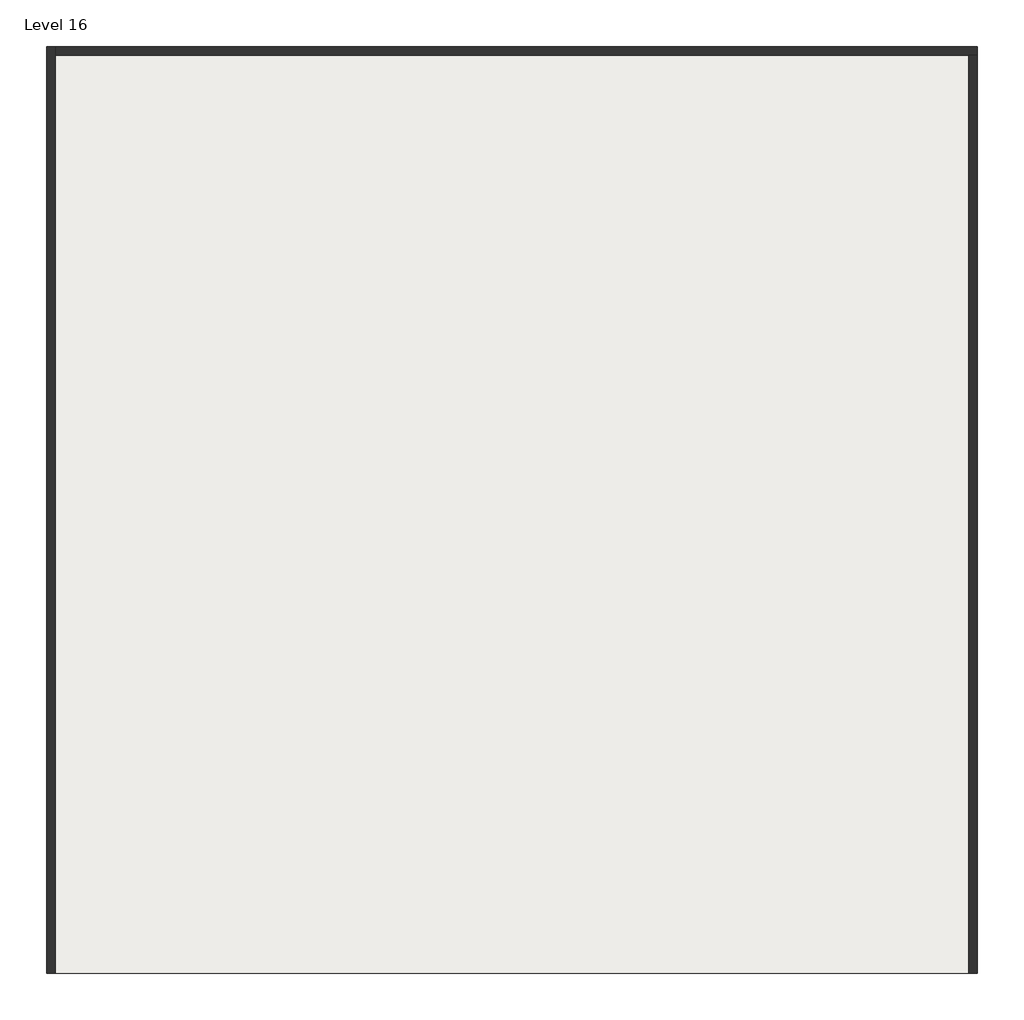
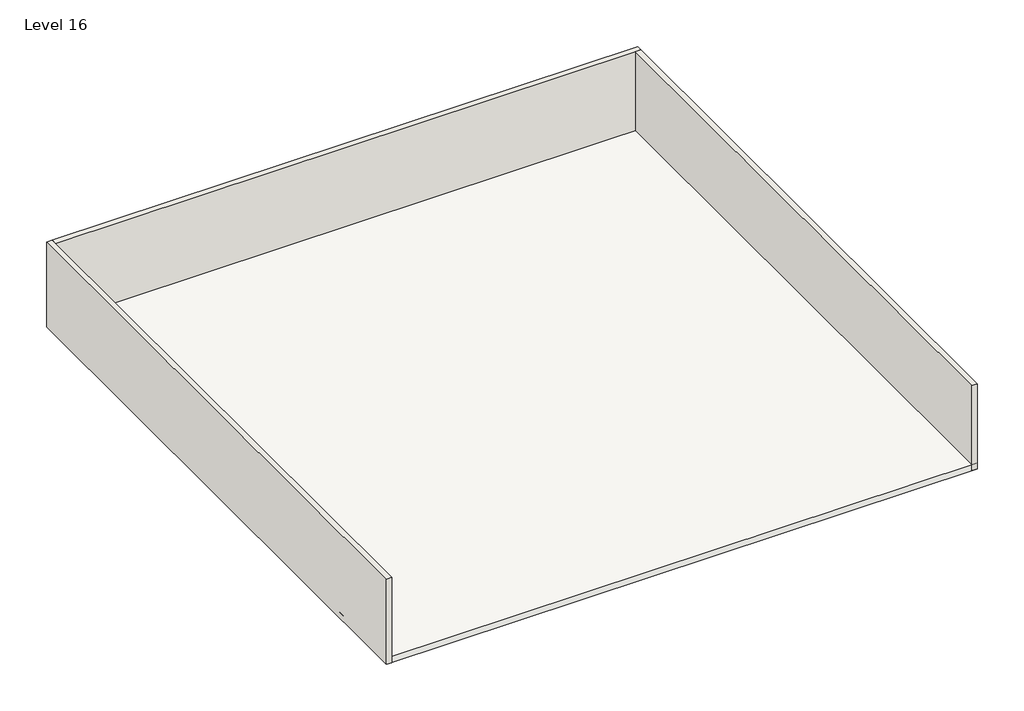
# One storey: 3 walls, 1 roof.
"""IFC4 building model written with IfcOpenShell, lengths in millimetres."""

from ifc_helpers import new_model, si_unit, frame, origin, place, context, project, spatial, polyline, outline, extrude, faceted_brep, element, save

model = new_model("IFC4")

# Units and contexts
model_context = context("Model", 3, world=origin())
ifc_project = project(units=[si_unit("LENGTHUNIT", "METRE", prefix="MILLI")], contexts=[model_context])

# Site, building, storey
site = spatial("IfcSite", under=ifc_project)
building = spatial("IfcBuilding", under=site)
storey = spatial("IfcBuildingStorey", under=building, Name="Level 16", Elevation=25984.2)

# Roof
placement = place(None, origin())
element("IfcRoof", 1, ObjectType="Generic - 9\"", at=placement, inside=storey, context=model_context, shape_type="SweptSolid", body=[
    extrude(outline(polyline([(-8934.7629849, 17755.0995758), (12604.4370151, 17755.0995758), (12604.4370151, -3682.5004242), (-8934.7629849, -3682.5004242), (-8934.7629849, 17755.0995758)])), frame((0.0, 0.0, 25984.2), z_axis=(0.0, 0.0, 1.0), x_axis=(1.0, 0.0, 0.0)), (0.0, 0.0, 1.0), 228.6),
])

# Walls
element("IfcWall", 2, ObjectType="outer wall", at=placement, inside=storey, context=model_context, shape_type="Brep", body=[
    faceted_brep([(-8731.5629849, -3682.5004242, 25984.2), (-8731.5629849, 17551.8995758, 25984.2), (-8731.5629849, 17755.0995758, 25984.2), (-8731.5629849, 17755.0995758, 29260.8), (-8731.5629849, 17551.8995758, 29260.8), (-8731.5629849, -3682.5004242, 29260.8), (-8934.7629849, -3682.5004242, 25984.2), (-8934.7629849, -3682.5004242, 29260.8), (-8934.7629849, 17755.0995758, 29260.8), (-8934.7629849, 17755.0995758, 25984.2)], [[[0, 1, 2, 3, 4, 5]], [[6, 7, 8, 9]], [[2, 1, 0, 6, 9]], [[5, 4, 3, 8, 7]], [[0, 5, 7, 6]], [[3, 2, 9, 8]]]),
])
element("IfcWall", 3, ObjectType="outer wall", at=placement, inside=storey, context=model_context, shape_type="Brep", body=[
    faceted_brep([(-8731.5629849, 17551.8995758, 25984.2), (12401.2370151, 17551.8995758, 25984.2), (12604.4370151, 17551.8995758, 25984.2), (12604.4370151, 17551.8995758, 29260.8), (12401.2370151, 17551.8995758, 29260.8), (-8731.5629849, 17551.8995758, 29260.8), (-8731.5629849, 17755.0995758, 25984.2), (-8731.5629849, 17755.0995758, 29260.8), (12604.4370151, 17755.0995758, 29260.8), (12604.4370151, 17755.0995758, 25984.2)], [[[0, 1, 2, 3, 4, 5]], [[6, 7, 8, 9]], [[2, 1, 0, 6, 9]], [[5, 4, 3, 8, 7]], [[0, 5, 7, 6]], [[3, 2, 9, 8]]]),
])
element("IfcWall", 4, ObjectType="outer wall", at=placement, inside=storey, context=model_context, shape_type="SweptSolid", body=[
    extrude(outline(polyline([(12604.4370151, 17551.8995758), (12604.4370151, -3682.5004242), (12401.2370151, -3682.5004242), (12401.2370151, 17551.8995758), (12604.4370151, 17551.8995758)])), frame((0.0, 0.0, 25984.2), z_axis=(0.0, 0.0, 1.0), x_axis=(1.0, 0.0, 0.0)), (0.0, 0.0, 1.0), 3276.6),
])

save(model, "model.ifc")

# Revit data of these elements
# Type "Generic - 9\""
#   Assembly Code = "B1020"
#   Layers, outside or top first: 0' - 9" no material (function 1)
# Type "outer wall"
#   Assembly Code = "B2010"
#   Layers, outside or top first: 0' - 8" "Copper" (function 1)
# Element 1 (IfcRoof, "Generic - 9\"")
#   built-in parameter 1001705 = 86 (stored number, unit not read)
#   built-in parameter 1001710 = 33615
#   Phase Created = New Construction
#   Materials on its faces: "Default Roof"
# Elements 2, 3, 4 (IfcWall, "outer wall")
#   Top Offset = 0' - 0"
#   Base Offset = 0' - 0"
#   Unconnected Height = 10' - 9"
#   wall height = 10' - 9"
#   Phase Created = New Construction
#   Base Constraint = Level 16
#   Materials on its faces: "Copper"
# Materials
#   "Copper": class "Metal", colour RGB 0 0 0, transparency 0, Description = "Copper, matte finish", Cost = 0
#   "Default Roof": colour RGB 88 101 114, transparency 0
